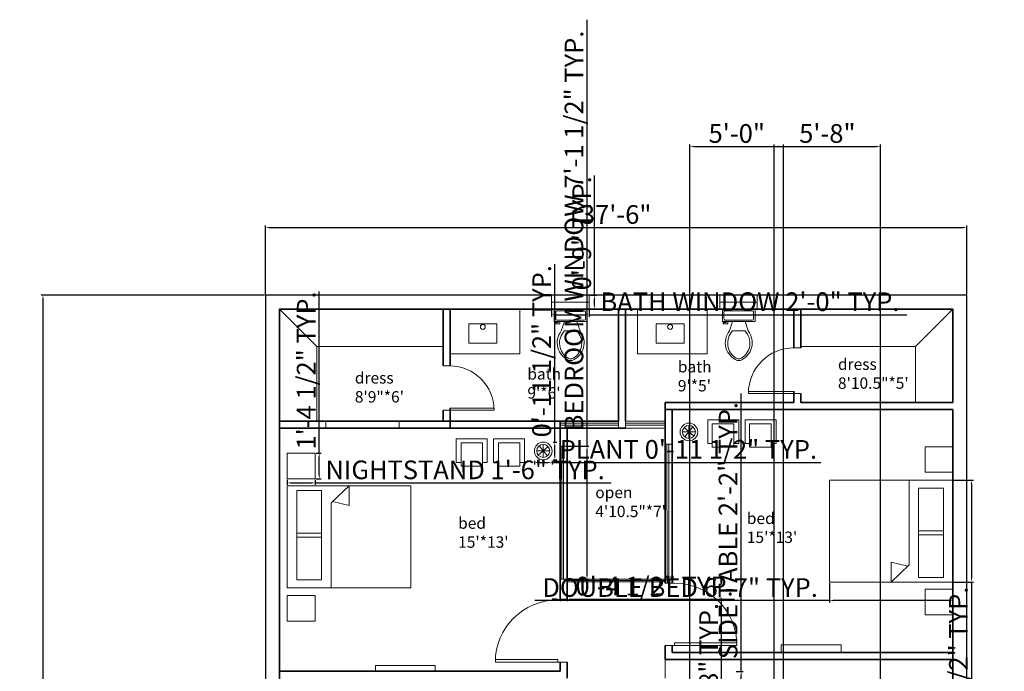
# Model space of a CAD drawing. Units: inches. Extents: x 3067 to 3879, y 3815 to 4813.
# Tile 3 of 3: x 3088 to 3719, y 4395 to 4813. Entities that reach past the tile are written whole.
import ezdxf

# ---------------------------------------------------------------- set-up
doc = ezdxf.new("R2010")
doc.units = ezdxf.units.IN
doc.linetypes.add('ACAD_ISO02W100', pattern=[15, 12, -3])
for name, color, linetype, lineweight in [('A-ANNO-DIMS', 2, 'Continuous', 18), ('A-AREA-IDEN', 7, 'Continuous', 18), ('A-DOOR', 3, 'Continuous', 18), ('A-EQPM', 8, 'Continuous', 18), ('A-FLOR-CASE', 8, 'Continuous', 20), ('A-FLOR-FIXT', 9, 'Continuous', 18), ('A-FLOR-OVHD', 8, 'ACAD_ISO02W100', 18), ('A-FURN', 8, 'Continuous', 18), ('A-GLAZ', 4, 'Continuous', 18), ('A-WALL', 7, 'Continuous', 35), ('C-PROP', 7, 'Continuous', 30)]:
    doc.layers.add(name, color=color, linetype=linetype, lineweight=lineweight)
doc.styles.get("Standard").update_dxf_attribs({"font": 'arial.ttf'})
doc.dimstyles.new('ISO-25', dxfattribs={"dimtxt": 12, "dimasz": 2.5, "dimexe": 1.25, "dimexo": 0.625, "dimtad": 1, "dimdec": 0, "dimlunit": 4, "dimtxsty": 'Standard', "dimcen": 2.5, "dimadec": 0, "dimazin": 0, "dimtfac": 1, "dimtdec": 0, "dimtmove": 0, "dimatfit": 3, "dimfxl": 1, "dimarcsym": 0})

# ---------------------------------------------------------------- blocks, each defined once
blk = doc.blocks.new('*U4')
for p, q in [((9.5, -6), (9.5, -2)), ((-10, -8.5), (-8, -8.5)), ((-10, -9.5), (-10, -8.5)), ((-7, -9.5), (-10, -9.5)), ((-8, -8.5), (-8, -8)), ((-7, -8), (-7, -9.5)), ((-4, -8), (-6, -14)), ((4, -8), (6, -14)), ((4, -14), (-4, -14))]:
    blk.add_line(p, q)
blk.add_lwpolyline([(10.5, -8), (10.5, 0), (-10.5, 0), (-10.5, -8)], close=True)
for points in [[(-9.5, -2), (-9.5, -6)], [(8.5, -1), (-8.5, -1)], [(-8.5, -7), (8.5, -7)]]:
    blk.add_lwpolyline(points)
for centre, radius, start, end in [((-8.62, -1.88), 0.884, 81.8699, 188.1301), ((-8.62, -6.12), 0.884, 171.8699, 278.1301), ((8.62, -1.88), 0.884, 351.8699, 98.1301), ((8.62, -6.12), 0.884, 261.8699, 8.1301), ((3.52, -21.58), 12.17, 141.46911, 247.97143), ((4.2, -21.82), 11.33, 136.36773, 238.94682), ((-3.52, -21.58), 12.17, 292.02843, 38.53071), ((-4.2, -21.82), 11.33, 301.05301, 43.63209), ((0, -27.88), 4, 245.73182, 294.26817), ((0, -29), 4, 254.86053, 285.13947)]:
    blk.add_arc(centre, radius, start, end)
blk = doc.blocks.new('*U2')
for p, q in [((0, 0), (0, -6)), ((40, 0), (40, -6))]:
    blk.add_line(p, q)
blk.add_lwpolyline([(0, 0), (0, 40), (1.75, 40), (1.75, 0)], close=True)
blk.add_arc((0, 0), 40, 0, 90)
blk = doc.blocks.new('*D7')
at = {"layer": 'A-ANNO-DIMS', "color": 0, "lineweight": -2, "transparency": 16777216}
for p, q in [((3245.41, 4636.9), (3245.41, 4680.99)), ((3695.41, 4636.9), (3695.41, 4680.99)), ((3247.91, 4679.74), (3692.91, 4679.74))]:
    blk.add_line(p, q, dxfattribs=at)
at = {"layer": 'A-ANNO-DIMS', "color": 0, "lineweight": 100, "transparency": 16777216}
for points in [[(3247.91, 4680.16), (3247.91, 4679.32), (3245.41, 4679.74)], [(3692.91, 4680.16), (3692.91, 4679.32), (3695.41, 4679.74)]]:
    blk.add_solid(points, dxfattribs=at)
at = {"layer": 'Defpoints', "color": 0, "lineweight": 100, "transparency": 16777216}
for p in [(3695.41, 4679.74), (3245.41, 4636.27), (3695.41, 4636.27)]:
    blk.add_point(p, dxfattribs=at)
at = {"layer": 'A-ANNO-DIMS', "color": 0, "transparency": 16777216, "insert": (3470.41, 4686.5), "char_height": 12, "attachment_point": 5}
blk.add_mtext('37\'-6"', dxfattribs=at)
blk = doc.blocks.new('*D8')
at = {"layer": 'A-ANNO-DIMS', "color": 0, "lineweight": -2, "transparency": 16777216}
for p, q in [((3244.78, 4636.27), (3101.49, 4636.27)), ((3102.74, 4633.77), (3102.74, 3918.77)), ((3244.78, 3916.27), (3101.49, 3916.27))]:
    blk.add_line(p, q, dxfattribs=at)
at = {"layer": 'A-ANNO-DIMS', "color": 0, "lineweight": 100, "transparency": 16777216}
for points in [[(3102.32, 4633.77), (3103.16, 4633.77), (3102.74, 4636.27)], [(3102.32, 3918.77), (3103.16, 3918.77), (3102.74, 3916.27)]]:
    blk.add_solid(points, dxfattribs=at)
at = {"layer": 'Defpoints', "color": 0, "lineweight": 100, "transparency": 16777216}
for p in [(3245.41, 4636.27), (3102.74, 3916.27), (3245.41, 3916.27)]:
    blk.add_point(p, dxfattribs=at)
at = {"layer": 'A-ANNO-DIMS', "color": 0, "transparency": 16777216, "insert": (3095.99, 4276.27), "char_height": 12, "attachment_point": 5, "rotation": 90}
blk.add_mtext("60'", dxfattribs=at)
blk = doc.blocks.new('CHAIR')
for p, q in [((0, 2.39), (0, 17.59)), ((0, 17.59), (19.86, 17.59)), ((19.86, 17.59), (19.86, 2.43)), ((3.13, 2.39), (0, 2.39)), ((19.86, 2.43), (16.92, 2.43))]:
    blk.add_line(p, q)
blk.add_lwpolyline([(3.13, 15.05), (16.92, 15.05), (16.92, 0), (3.13, 0)], close=True)
blk = doc.blocks.new('BED-DOUBLE')
for p, q in [((28.12, 54.48), (39.62, 65.45)), ((39.62, 65.45), (39.62, 52.71)), ((28.12, 0), (28.12, 54.48)), ((39.62, 52.71), (29.02, 55.33))]:
    blk.add_line(p, q)
for points in [[(0, 0), (79.24, 0), (79.24, 65.45), (0, 65.45)], [(6.11, 32.53), (21.99, 32.53), (21.99, 62.5), (6.11, 62.5)], [(6.11, 5.18), (21.99, 5.18), (21.99, 35.15), (6.11, 35.15)]]:
    blk.add_lwpolyline(points, close=True)
blk = doc.blocks.new('NIGHTSTAND')
blk.add_lwpolyline([(0, 0), (17.91, 0), (17.91, 16.38), (0, 16.38)], close=True)
blk = doc.blocks.new('PLANT-ROUND')
for p, q in [((1.02, 1.45), (7.33, 6.97)), ((6.87, 0.97), (1.63, 7.51)), ((4.2, 8.39), (4.2, 0)), ((0, 4.21), (8.39, 4.21))]:
    blk.add_line(p, q)
for radius in [5.68, 4.19]:
    blk.add_circle((4.19, 4.19), radius)
blk = doc.blocks.new('VANITY-BASIN')
for points in [[(0, 28.58), (44.74, 28.58), (44.74, 0), (0, 0)], [(11.93, 6.65), (29.93, 6.65), (29.93, 19.14), (11.93, 19.14)]]:
    blk.add_lwpolyline(points, close=True)
blk.add_circle((20.98, 17.18), 1.58)
blk = doc.blocks.new('WIN-BATH-24')
for p, q in [((0, 0), (0, 9)), ((24, 0), (24, 9)), ((0, 4.5), (24, 4.5))]:
    blk.add_line(p, q)
blk = doc.blocks.new('WIN-BEDROOM')
for p, q in [((1.09, 85.44), (1.21, 0)), ((2.25, 85.44), (2.25, 0))]:
    blk.add_line(p, q)
blk.add_lwpolyline([(0, 85.44), (4.5, 85.44), (4.5, 0), (0, 0)], close=True)
blk = doc.blocks.new('*D21')
at = {"layer": 'A-ANNO-DIMS', "color": 0, "lineweight": -2, "transparency": 16777216}
for p, q in [((3538.08, 4308.43), (3538.08, 4442)), ((3535.73, 4308.43), (3539.33, 4308.43)), ((3538.08, 4291.07), (3538.08, 4305.93)), ((3535.73, 4288.57), (3539.33, 4288.57))]:
    blk.add_line(p, q, dxfattribs=at)
at = {"layer": 'A-ANNO-DIMS', "color": 0, "lineweight": 100, "transparency": 16777216}
for points in [[(3537.67, 4305.93), (3538.5, 4305.93), (3538.08, 4308.43)], [(3537.67, 4291.07), (3538.5, 4291.07), (3538.08, 4288.57)]]:
    blk.add_solid(points, dxfattribs=at)
at = {"layer": 'Defpoints', "color": 0, "lineweight": 100, "transparency": 16777216}
for p in [(3535.11, 4308.43), (3538.08, 4308.43), (3535.11, 4288.57)]:
    blk.add_point(p, dxfattribs=at)
at = {"layer": 'A-ANNO-DIMS', "color": 0, "transparency": 16777216, "insert": (3531.25, 4376.46), "char_height": 12, "attachment_point": 5, "rotation": 90}
blk.add_mtext('CHAIR 1\'-8" TYP.', dxfattribs=at)
blk = doc.blocks.new('*D23')
at = {"layer": 'A-ANNO-DIMS', "color": 0, "lineweight": -2, "transparency": 16777216}
for p, q in [((3259.36, 4517.78), (3259.36, 4514.47)), ((3261.86, 4515.72), (3274.78, 4515.72)), ((3277.28, 4517.78), (3277.28, 4514.47)), ((3277.28, 4515.72), (3467.22, 4515.72))]:
    blk.add_line(p, q, dxfattribs=at)
at = {"layer": 'A-ANNO-DIMS', "color": 0, "lineweight": 100, "transparency": 16777216}
for points in [[(3261.86, 4516.13), (3261.86, 4515.3), (3259.36, 4515.72)], [(3274.78, 4516.13), (3274.78, 4515.3), (3277.28, 4515.72)]]:
    blk.add_solid(points, dxfattribs=at)
at = {"layer": 'Defpoints', "color": 0, "lineweight": 100, "transparency": 16777216}
for p in [(3259.36, 4518.4), (3277.28, 4518.4), (3277.28, 4515.72)]:
    blk.add_point(p, dxfattribs=at)
at = {"layer": 'A-ANNO-DIMS', "color": 0, "transparency": 16777216, "insert": (3373.5, 4522.55), "char_height": 12, "attachment_point": 5}
blk.add_mtext('NIGHTSTAND 1\'-6" TYP.', dxfattribs=at)
blk = doc.blocks.new('*D24')
at = {"layer": 'A-ANNO-DIMS', "color": 0, "lineweight": -2, "transparency": 16777216}
for p, q in [((3279.96, 4534.79), (3279.96, 4638.51)), ((3277.9, 4534.79), (3281.21, 4534.79)), ((3279.96, 4520.9), (3279.96, 4532.29)), ((3277.9, 4518.4), (3281.21, 4518.4))]:
    blk.add_line(p, q, dxfattribs=at)
at = {"layer": 'A-ANNO-DIMS', "color": 0, "lineweight": 100, "transparency": 16777216}
for points in [[(3279.55, 4532.29), (3280.38, 4532.29), (3279.96, 4534.79)], [(3279.55, 4520.9), (3280.38, 4520.9), (3279.96, 4518.4)]]:
    blk.add_solid(points, dxfattribs=at)
at = {"layer": 'Defpoints', "color": 0, "lineweight": 100, "transparency": 16777216}
for p in [(3277.28, 4534.79), (3279.96, 4534.79), (3277.28, 4518.4)]:
    blk.add_point(p, dxfattribs=at)
at = {"layer": 'A-ANNO-DIMS', "color": 0, "transparency": 16777216, "insert": (3273.13, 4587.9), "char_height": 12, "attachment_point": 5, "rotation": 90}
blk.add_mtext('1\'-4 1/2" TYP.', dxfattribs=at)
blk = doc.blocks.new('*D29')
at = {"layer": 'A-ANNO-DIMS', "color": 0, "lineweight": -2, "transparency": 16777216}
for p, q in [((3550.59, 4394.65), (3550.59, 4573.04)), ((3547.3, 4394.65), (3551.84, 4394.65)), ((3550.59, 4371.05), (3550.59, 4392.15)), ((3547.3, 4368.55), (3551.84, 4368.55))]:
    blk.add_line(p, q, dxfattribs=at)
at = {"layer": 'A-ANNO-DIMS', "color": 0, "lineweight": 100, "transparency": 16777216}
for points in [[(3550.17, 4392.15), (3551.01, 4392.15), (3550.59, 4394.65)], [(3550.17, 4371.05), (3551.01, 4371.05), (3550.59, 4368.55)]]:
    blk.add_solid(points, dxfattribs=at)
at = {"layer": 'Defpoints', "color": 0, "lineweight": 100, "transparency": 16777216}
for p in [(3546.67, 4394.65), (3550.59, 4394.65), (3546.67, 4368.55)]:
    blk.add_point(p, dxfattribs=at)
at = {"layer": 'A-ANNO-DIMS', "color": 0, "transparency": 16777216, "insert": (3543.76, 4485.1), "char_height": 12, "attachment_point": 5, "rotation": 90}
blk.add_mtext('SIDE TABLE 2\'-2" TYP.', dxfattribs=at)
blk = doc.blocks.new('*D35')
at = {"layer": 'A-ANNO-DIMS', "color": 0, "lineweight": -2, "transparency": 16777216}
for p, q in [((3607.17, 4451.42), (3607.17, 4438.91)), ((3686.41, 4451.42), (3686.41, 4438.91)), ((3607.17, 4440.16), (3418.14, 4440.16)), ((3683.91, 4440.16), (3609.67, 4440.16))]:
    blk.add_line(p, q, dxfattribs=at)
at = {"layer": 'A-ANNO-DIMS', "color": 0, "lineweight": 100, "transparency": 16777216}
for points in [[(3609.67, 4440.58), (3609.67, 4439.74), (3607.17, 4440.16)], [(3683.91, 4440.58), (3683.91, 4439.74), (3686.41, 4440.16)]]:
    blk.add_solid(points, dxfattribs=at)
at = {"layer": 'Defpoints', "color": 0, "lineweight": 100, "transparency": 16777216}
for p in [(3607.17, 4452.05), (3686.41, 4452.05), (3607.17, 4440.16)]:
    blk.add_point(p, dxfattribs=at)
at = {"layer": 'A-ANNO-DIMS', "color": 0, "transparency": 16777216, "insert": (3511.41, 4446.99), "char_height": 12, "attachment_point": 5}
blk.add_mtext('DOUBLE BED 6\'-7" TYP.', dxfattribs=at)
blk = doc.blocks.new('*D36')
at = {"layer": 'A-ANNO-DIMS', "color": 0, "lineweight": -2, "transparency": 16777216}
for p, q in [((3687.03, 4517.5), (3699.54, 4517.5)), ((3698.29, 4515), (3698.29, 4454.55)), ((3687.03, 4452.05), (3699.54, 4452.05)), ((3698.29, 4452.05), (3698.29, 4347.19))]:
    blk.add_line(p, q, dxfattribs=at)
at = {"layer": 'A-ANNO-DIMS', "color": 0, "lineweight": 100, "transparency": 16777216}
for points in [[(3697.88, 4515), (3698.71, 4515), (3698.29, 4517.5)], [(3697.88, 4454.55), (3698.71, 4454.55), (3698.29, 4452.05)]]:
    blk.add_solid(points, dxfattribs=at)
at = {"layer": 'Defpoints', "color": 0, "lineweight": 100, "transparency": 16777216}
for p in [(3686.41, 4517.5), (3686.41, 4452.05), (3698.29, 4452.05)]:
    blk.add_point(p, dxfattribs=at)
at = {"layer": 'A-ANNO-DIMS', "color": 0, "transparency": 16777216, "insert": (3691.46, 4398.37), "char_height": 12, "attachment_point": 5, "rotation": 90}
blk.add_mtext('5\'-5 1/2" TYP.', dxfattribs=at)
blk = doc.blocks.new('*D37')
at = {"layer": 'A-ANNO-DIMS', "color": 0, "lineweight": -2, "transparency": 16777216}
for p, q in [((3417.98, 4529.94), (3417.98, 4527.61)), ((3420.48, 4528.86), (3426.84, 4528.86)), ((3429.34, 4529.94), (3429.34, 4527.61)), ((3429.34, 4528.86), (3601.61, 4528.86))]:
    blk.add_line(p, q, dxfattribs=at)
at = {"layer": 'A-ANNO-DIMS', "color": 0, "lineweight": 100, "transparency": 16777216}
for points in [[(3420.48, 4529.28), (3420.48, 4528.44), (3417.98, 4528.86)], [(3426.84, 4529.28), (3426.84, 4528.44), (3429.34, 4528.86)]]:
    blk.add_solid(points, dxfattribs=at)
at = {"layer": 'Defpoints', "color": 0, "lineweight": 100, "transparency": 16777216}
for p in [(3417.98, 4530.56), (3429.34, 4530.56), (3429.34, 4528.86)]:
    blk.add_point(p, dxfattribs=at)
at = {"layer": 'A-ANNO-DIMS', "color": 0, "transparency": 16777216, "insert": (3516.72, 4535.69), "char_height": 12, "attachment_point": 5}
blk.add_mtext('PLANT 0\'-11 1/2" TYP.', dxfattribs=at)
blk = doc.blocks.new('*D38')
at = {"layer": 'A-ANNO-DIMS', "color": 0, "lineweight": -2, "transparency": 16777216}
for p, q in [((3431.04, 4541.92), (3431.04, 4656.1)), ((3429.96, 4541.92), (3432.29, 4541.92)), ((3431.04, 4533.06), (3431.04, 4539.42)), ((3429.96, 4530.56), (3432.29, 4530.56))]:
    blk.add_line(p, q, dxfattribs=at)
at = {"layer": 'A-ANNO-DIMS', "color": 0, "lineweight": 100, "transparency": 16777216}
for points in [[(3430.62, 4539.42), (3431.46, 4539.42), (3431.04, 4541.92)], [(3430.62, 4533.06), (3431.46, 4533.06), (3431.04, 4530.56)]]:
    blk.add_solid(points, dxfattribs=at)
at = {"layer": 'Defpoints', "color": 0, "lineweight": 100, "transparency": 16777216}
for p in [(3429.34, 4541.92), (3431.04, 4541.92), (3429.34, 4530.56)]:
    blk.add_point(p, dxfattribs=at)
at = {"layer": 'A-ANNO-DIMS', "color": 0, "transparency": 16777216, "insert": (3424.21, 4600.26), "char_height": 12, "attachment_point": 5, "rotation": 90}
blk.add_mtext('0\'-11 1/2" TYP.', dxfattribs=at)
blk = doc.blocks.new('*D39')
at = {"layer": 'A-ANNO-DIMS', "color": 0, "lineweight": -2, "transparency": 16777216}
for p, q in [((3429.01, 4626.65), (3429.01, 4622.42)), ((3431.51, 4623.67), (3450.51, 4623.67)), ((3453.01, 4626.65), (3453.01, 4622.42)), ((3453.01, 4623.67), (3656.95, 4623.67))]:
    blk.add_line(p, q, dxfattribs=at)
at = {"layer": 'A-ANNO-DIMS', "color": 0, "lineweight": 100, "transparency": 16777216}
for points in [[(3431.51, 4624.09), (3431.51, 4623.26), (3429.01, 4623.67)], [(3450.51, 4624.09), (3450.51, 4623.26), (3453.01, 4623.67)]]:
    blk.add_solid(points, dxfattribs=at)
at = {"layer": 'Defpoints', "color": 0, "lineweight": 100, "transparency": 16777216}
for p in [(3429.01, 4627.27), (3453.01, 4627.27), (3453.01, 4623.67)]:
    blk.add_point(p, dxfattribs=at)
at = {"layer": 'A-ANNO-DIMS', "color": 0, "transparency": 16777216, "insert": (3556.23, 4630.51), "char_height": 12, "attachment_point": 5}
blk.add_mtext('BATH WINDOW 2\'-0" TYP.', dxfattribs=at)
blk = doc.blocks.new('*D40')
at = {"layer": 'A-ANNO-DIMS', "color": 0, "lineweight": -2, "transparency": 16777216}
for p, q in [((3456.61, 4636.27), (3456.61, 4713.17)), ((3453.63, 4636.27), (3457.86, 4636.27)), ((3456.61, 4629.77), (3456.61, 4633.77)), ((3453.63, 4627.27), (3457.86, 4627.27))]:
    blk.add_line(p, q, dxfattribs=at)
at = {"layer": 'A-ANNO-DIMS', "color": 0, "lineweight": 100, "transparency": 16777216}
for points in [[(3456.19, 4633.77), (3457.03, 4633.77), (3456.61, 4636.27)], [(3456.19, 4629.77), (3457.03, 4629.77), (3456.61, 4627.27)]]:
    blk.add_solid(points, dxfattribs=at)
at = {"layer": 'Defpoints', "color": 0, "lineweight": 100, "transparency": 16777216}
for p in [(3453.01, 4636.27), (3456.61, 4636.27), (3453.01, 4627.27)]:
    blk.add_point(p, dxfattribs=at)
at = {"layer": 'A-ANNO-DIMS', "color": 0, "transparency": 16777216, "insert": (3449.86, 4675.97), "char_height": 12, "attachment_point": 5, "rotation": 90}
blk.add_mtext('0\'-9" TYP.', dxfattribs=at)
blk = doc.blocks.new('*D41')
at = {"layer": 'A-ANNO-DIMS', "color": 0, "lineweight": -2, "transparency": 16777216}
for p, q in [((3451.72, 4539.32), (3451.72, 4813.14)), ((3439.53, 4539.32), (3452.97, 4539.32)), ((3451.72, 4456.39), (3451.72, 4536.82)), ((3439.53, 4453.89), (3452.97, 4453.89))]:
    blk.add_line(p, q, dxfattribs=at)
at = {"layer": 'A-ANNO-DIMS', "color": 0, "lineweight": 100, "transparency": 16777216}
for points in [[(3451.31, 4536.82), (3452.14, 4536.82), (3451.72, 4539.32)], [(3451.31, 4456.39), (3452.14, 4456.39), (3451.72, 4453.89)]]:
    blk.add_solid(points, dxfattribs=at)
at = {"layer": 'Defpoints', "color": 0, "lineweight": 100, "transparency": 16777216}
for p in [(3438.91, 4539.32), (3451.72, 4539.32), (3438.91, 4453.89)]:
    blk.add_point(p, dxfattribs=at)
at = {"layer": 'A-ANNO-DIMS', "color": 0, "transparency": 16777216, "insert": (3444.89, 4677.48), "char_height": 12, "attachment_point": 5, "rotation": 90}
blk.add_mtext('BEDROOM WINDOW 7\'-1 1/2" TYP.', dxfattribs=at)
blk = doc.blocks.new('*D42')
at = {"layer": 'A-ANNO-DIMS', "color": 0, "lineweight": -2, "transparency": 16777216}
for p, q in [((3434.41, 4453.26), (3434.41, 4439.82)), ((3438.91, 4453.26), (3438.91, 4439.82)), ((3431.91, 4441.07), (3429.41, 4441.07)), ((3434.41, 4441.07), (3438.91, 4441.07)), ((3441.41, 4441.07), (3546.27, 4441.07))]:
    blk.add_line(p, q, dxfattribs=at)
at = {"layer": 'A-ANNO-DIMS', "color": 0, "lineweight": 100, "transparency": 16777216}
for points in [[(3431.91, 4441.49), (3431.91, 4440.65), (3434.41, 4441.07)], [(3441.41, 4441.49), (3441.41, 4440.65), (3438.91, 4441.07)]]:
    blk.add_solid(points, dxfattribs=at)
at = {"layer": 'Defpoints', "color": 0, "lineweight": 100, "transparency": 16777216}
for p in [(3434.41, 4453.89), (3438.91, 4453.89), (3438.91, 4441.07)]:
    blk.add_point(p, dxfattribs=at)
at = {"layer": 'A-ANNO-DIMS', "color": 0, "transparency": 16777216, "insert": (3495.09, 4447.9), "char_height": 12, "attachment_point": 5}
blk.add_mtext('0\'-4 1/2" TYP.', dxfattribs=at)
blk = doc.blocks.new('*D47')
at = {"layer": 'A-ANNO-DIMS', "color": 0, "lineweight": -2, "transparency": 16777216}
for p, q in [((3571.86, 4180.9), (3571.86, 4733.02)), ((3574.36, 4731.77), (3637.41, 4731.77)), ((3639.91, 4180.9), (3639.91, 4733.02))]:
    blk.add_line(p, q, dxfattribs=at)
at = {"layer": 'A-ANNO-DIMS', "color": 0, "lineweight": 100, "transparency": 16777216}
for points in [[(3574.36, 4732.19), (3574.36, 4731.36), (3571.86, 4731.77)], [(3637.41, 4732.19), (3637.41, 4731.36), (3639.91, 4731.77)]]:
    blk.add_solid(points, dxfattribs=at)
at = {"layer": 'Defpoints', "color": 0, "lineweight": 100, "transparency": 16777216}
for p in [(3639.91, 4731.77), (3571.86, 4180.27), (3639.91, 4180.27)]:
    blk.add_point(p, dxfattribs=at)
at = {"layer": 'A-ANNO-DIMS', "color": 0, "transparency": 16777216, "insert": (3605.89, 4738.52), "char_height": 12, "attachment_point": 5}
blk.add_mtext('5\'-8"', dxfattribs=at)
blk = doc.blocks.new('*D50')
at = {"layer": 'A-ANNO-DIMS', "color": 0, "lineweight": -2, "transparency": 16777216}
for p, q in [((3517.72, 4129.9), (3517.72, 4733.02)), ((3520.22, 4731.77), (3575.32, 4731.77)), ((3577.82, 4129.9), (3577.82, 4733.02))]:
    blk.add_line(p, q, dxfattribs=at)
at = {"layer": 'A-ANNO-DIMS', "color": 0, "lineweight": 100, "transparency": 16777216}
for points in [[(3520.22, 4732.19), (3520.22, 4731.36), (3517.72, 4731.77)], [(3575.32, 4732.19), (3575.32, 4731.36), (3577.82, 4731.77)]]:
    blk.add_solid(points, dxfattribs=at)
at = {"layer": 'Defpoints', "color": 0, "lineweight": 100, "transparency": 16777216}
for p in [(3577.82, 4731.77), (3517.72, 4129.27), (3577.82, 4129.27)]:
    blk.add_point(p, dxfattribs=at)
at = {"layer": 'A-ANNO-DIMS', "color": 0, "transparency": 16777216, "insert": (3547.77, 4738.52), "char_height": 12, "attachment_point": 5}
blk.add_mtext('5\'-0"', dxfattribs=at)

msp = doc.modelspace()

# ---------------------------------------------------------------- linework, layer by layer
at = {"layer": 'A-EQPM'}
for points in [[(3576.16, 4406.77), (3614.64, 4406.77), (3614.64, 4411.85), (3576.16, 4411.85)], [(3316.12, 4394.77), (3354.25, 4394.77), (3354.25, 4398.57), (3316.12, 4398.57)]]:
    msp.add_lwpolyline(points, close=True, dxfattribs=at)
at = {"layer": 'A-FLOR-CASE'}
for p, q in [((3278.41, 4603.27), (3254.41, 4627.27)), ((3359.41, 4627.27), (3359.41, 4603.27)), ((3588.91, 4627.27), (3588.91, 4603.27)), ((3662.41, 4603.27), (3686.41, 4627.27)), ((3278.41, 4555.6), (3278.41, 4603.27)), ((3359.41, 4603.27), (3278.41, 4603.27)), ((3588.91, 4603.27), (3662.41, 4603.27)), ((3662.41, 4567.27), (3662.41, 4603.27)), ((3686.41, 4567.27), (3662.41, 4567.27)), ((3278.41, 4556.68), (3278.41, 4555.27))]:
    msp.add_line(p, q, dxfattribs=at)
at = {"layer": 'A-FLOR-OVHD'}
msp.add_line((3501.91, 4402.27), (3501.91, 4222.27), dxfattribs=at)
at = {"layer": 'A-GLAZ'}
for p, q in [((3434.41, 4554.04), (3471.91, 4554.04)), ((3471.91, 4555.27), (3471.91, 4550.77)), ((3476.41, 4555.27), (3501.91, 4555.27)), ((3476.41, 4555.27), (3476.41, 4550.77)), ((3476.41, 4554.04), (3501.91, 4554.04)), ((3434.41, 4552.83), (3471.91, 4552.83)), ((3476.41, 4552.83), (3501.91, 4552.83)), ((3476.41, 4550.77), (3501.91, 4550.77)), ((3438.91, 4453.05), (3501.91, 4453.05))]:
    msp.add_line(p, q, dxfattribs=at)
for points in [[(3284.1, 4555.27), (3331.23, 4555.27), (3331.23, 4550.77), (3284.1, 4550.77)], [(3501.91, 4452.21), (3438.91, 4452.21), (3438.91, 4453.89), (3501.91, 4453.89)]]:
    msp.add_lwpolyline(points, close=True, dxfattribs=at)
at = {"layer": 'A-WALL'}
for p, q in [((3254.41, 4627.27), (3359.41, 4627.27)), ((3359.41, 4627.27), (3359.41, 4590.85)), ((3363.91, 4627.27), (3363.91, 4590.85)), ((3363.91, 4627.27), (3471.91, 4627.27)), ((3471.91, 4627.27), (3471.91, 4555.27)), ((3476.41, 4627.27), (3476.41, 4555.27)), ((3476.41, 4627.27), (3584.41, 4627.27)), ((3584.41, 4627.27), (3584.41, 4602.48)), ((3588.91, 4627.27), (3588.91, 4602.48)), ((3588.91, 4627.27), (3686.41, 4627.27)), ((3584.41, 4574.48), (3584.41, 4567.27)), ((3588.91, 4573.2), (3588.91, 4567.27)), ((3584.41, 4567.27), (3501.91, 4567.27)), ((3501.91, 4562.77), (3501.91, 4567.27)), ((3588.91, 4567.27), (3686.41, 4567.27)), ((3359.41, 4562.42), (3359.41, 4555.27)), ((3363.91, 4563.66), (3363.91, 4550.77)), ((3588.91, 4562.77), (3501.91, 4562.77)), ((3501.91, 4451.29), (3501.91, 4562.77)), ((3506.41, 4451.29), (3506.41, 4562.77)), ((3588.91, 4562.77), (3686.41, 4562.77)), ((3686.41, 4562.77), (3686.41, 4406.77)), ((3359.41, 4555.27), (3254.41, 4555.27)), ((3471.91, 4555.27), (3359.41, 4555.27)), ((3434.41, 4545.06), (3434.41, 4555.27)), ((3363.91, 4550.77), (3254.41, 4550.77)), ((3254.41, 4550.77), (3254.41, 4394.77)), ((3476.41, 4550.77), (3359.41, 4550.77)), ((3434.41, 4440.62), (3434.41, 4550.77)), ((3438.91, 4440.62), (3438.91, 4550.77)), ((3501.91, 4402.27), (3501.91, 4411.29)), ((3506.41, 4406.77), (3506.41, 4411.29)), ((3686.41, 4402.27), (3501.91, 4402.27)), ((3686.41, 4406.77), (3506.41, 4406.77)), ((3686.41, 4402.27), (3686.41, 4222.27)), ((3434.41, 4394.77), (3434.41, 4400.62)), ((3438.91, 4390.27), (3438.91, 4400.62)), ((3254.41, 4394.77), (3422.41, 4394.77)), ((3254.41, 4394.77), (3434.41, 4394.77))]:
    msp.add_line(p, q, dxfattribs=at)
for points in [[(3686.41, 4567.27), (3686.41, 4627.27), (3254.41, 4627.27), (3254.41, 3925.27), (3494.41, 3925.27)], [(3686.41, 3925.27), (3686.41, 4562.77)]]:
    msp.add_lwpolyline(points, dxfattribs=at)
at = {"layer": 'C-PROP'}
msp.add_lwpolyline([(3245.41, 3916.27), (3695.41, 3916.27), (3695.41, 4636.27), (3245.41, 4636.27)], close=True, dxfattribs=at)

# ---------------------------------------------------------------- block references
at = {"layer": 'A-DOOR'}
for p, xscale, yscale, zscale, rotation in [((3584.52, 4573.2), 0.7320240099699031, 0.7320240099699031, 0.7320240099699031, 90), ((3363.67, 4562.42), -0.7108348998799947, 0.7108348998799947, 0.7108348998799947, 270)]:
    msp.add_blockref('*U2', p, dxfattribs=dict(at, xscale=xscale, yscale=yscale, zscale=zscale, rotation=rotation))
at = {"layer": 'A-DOOR', "xscale": -1, "rotation": 270}
msp.add_blockref('*U2', (3507.91, 4411.29), dxfattribs=at)
at = {"layer": 'A-DOOR', "rotation": 90}
msp.add_blockref('*U2', (3432.91, 4400.62), dxfattribs=at)
at = {"layer": 'A-FLOR-FIXT'}
for name, p in [('VANITY-BASIN', (3363.91, 4598.69)), ('*U4', (3441.22, 4627.27)), ('VANITY-BASIN', (3484.04, 4598.69)), ('*U4', (3549.06, 4627.27))]:
    msp.add_blockref(name, p, dxfattribs=at)
at = {"layer": 'A-FURN', "extrusion": (0, 0, -1), "zscale": -1}
for name, p in [('PLANT-ROUND', (-3521.3, 4544.24)), ('CHAIR', (-3549, 4538.6)), ('CHAIR', (-3572.95, 4538.6))]:
    msp.add_blockref(name, p, dxfattribs=at)
at = {"layer": 'A-FURN'}
for name, p in [('CHAIR', (3367.81, 4526.4)), ('CHAIR', (3391.76, 4526.4)), ('PLANT-ROUND', (3419.46, 4532.05)), ('NIGHTSTAND', (3259.36, 4518.4)), ('BED-DOUBLE', (3259.43, 4448.4)), ('NIGHTSTAND', (3259.36, 4426.98))]:
    msp.add_blockref(name, p, dxfattribs=at)
at = {"layer": 'A-FURN', "rotation": 180}
for name, p in [('NIGHTSTAND', (3686.47, 4538.92)), ('BED-DOUBLE', (3686.41, 4517.5)), ('NIGHTSTAND', (3686.47, 4447.5))]:
    msp.add_blockref(name, p, dxfattribs=at)
at = {"layer": 'A-GLAZ'}
for name, p in [('WIN-BATH-24', (3429.01, 4627.27)), ('WIN-BATH-24', (3536.92, 4627.27)), ('WIN-BEDROOM', (3434.41, 4453.89)), ('WIN-BEDROOM', (3501.91, 4455.14))]:
    msp.add_blockref(name, p, dxfattribs=at)

# ---------------------------------------------------------------- texts
at = {"layer": 'A-AREA-IDEN', "char_height": 7.308, "attachment_point": 1}
for s, insert in [("bath\\P9'*5'", (3509.98, 4593.95)), ('dress\\P8\'10.5"*5\'', (3612.67, 4595.61)), ('dress\\P8\'9"*6\'', (3302.78, 4586.82)), ("bath\\P9'*6'", (3413.46, 4589.34)), ('open\\P4\'10.5"*7\'', (3457.02, 4513.24)), ("bed\\P15'*13'", (3554.23, 4496.64)), ("bed\\P15'*13'", (3369.05, 4493.57))]:
    msp.add_mtext_dynamic_manual_height_columns(s, width=269.495, gutter_width=36.54, heights=[0], dxfattribs=dict(at, insert=insert))

# ---------------------------------------------------------------- dimensions: what is measured, and where the dimension line sits
at = {"layer": 'A-ANNO-DIMS'}
for base, p1, p2, angle, text, picture, middle in [((3451.72, 4539.32), (3438.91, 4453.89), (3438.91, 4539.32), 90, 'BEDROOM WINDOW <> TYP.', '*D41', (3444.89, 4677.48)), ((3456.61, 4636.27), (3453.01, 4627.27), (3453.01, 4636.27), 90, '<> TYP.', '*D40', (3449.86, 4675.97)), ((3431.04, 4541.92), (3429.34, 4530.56), (3429.34, 4541.92), 90, '<> TYP.', '*D38', (3424.21, 4600.26)), ((3279.96, 4534.79), (3277.28, 4518.4), (3277.28, 4534.79), 90, '<> TYP.', '*D24', (3273.13, 4587.9)), ((3550.59, 4394.65), (3546.67, 4368.55), (3546.67, 4394.65), 90, 'SIDE TABLE <> TYP.', '*D29', (3543.76, 4485.1)), ((3698.2935, 4452.0456), (3686.4073, 4517.4994), (3686.4073, 4452.0456), 270, '<> TYP.', '*D36', (3691.4639, 4398.3667)), ((3607.17, 4440.16), (3686.41, 4452.05), (3607.17, 4452.05), 180, 'DOUBLE BED <> TYP.', '*D35', (3511.41, 4446.99)), ((3538.08, 4308.43), (3535.11, 4288.57), (3535.11, 4308.43), 90, 'CHAIR <> TYP.', '*D21', (3531.25, 4376.46))]:
    dim = msp.add_linear_dim(base=base, p1=p1, p2=p2, angle=angle, text=text, dimstyle='ISO-25', override={"dimdec": 1, "dimlfac": 1, "dimrnd": 0, "dimzin": 1, "dimdsep": 46, "dimlunit": 4, "dimfrac": 2}, dxfattribs=at)
    dim.commit()
    dim.dimension.update_dxf_attribs({"geometry": picture, "text_midpoint": middle})
for base, p1, p2, override, picture, middle in [((3577.82, 4731.77), (3517.72, 4129.27), (3577.82, 4129.27), {"dimdec": 1, "dimlfac": 1, "dimrnd": 0, "dimzin": 1, "dimdsep": 46, "dimlunit": 4, "dimfrac": 2}, '*D50', (3547.77, 4738.52)), ((3639.9073, 4731.7725), (3571.865, 4180.2725), (3639.9073, 4180.2725), {"dimdec": 1, "dimlfac": 1, "dimrnd": 0, "dimzin": 1, "dimdsep": 46, "dimlunit": 4, "dimfrac": 2}, '*D47', (3605.8862, 4738.5244)), ((3695.41, 4679.74), (3245.41, 4636.27), (3695.41, 4636.27), {"dimclrd": 0, "dimclre": 0, "dimclrt": 0}, '*D7', (3470.41, 4686.5))]:
    dim = msp.add_linear_dim(base=base, p1=p1, p2=p2, dimstyle='ISO-25', override=override, dxfattribs=at)
    dim.commit()
    dim.dimension.update_dxf_attribs({"geometry": picture, "text_midpoint": middle})
for base, p1, p2, text, picture, middle in [((3453.01, 4623.67), (3429.01, 4627.27), (3453.01, 4627.27), 'BATH WINDOW <> TYP.', '*D39', (3556.23, 4630.51)), ((3429.34, 4528.86), (3417.98, 4530.56), (3429.34, 4530.56), 'PLANT <> TYP.', '*D37', (3516.72, 4535.69)), ((3277.28, 4515.72), (3259.36, 4518.4), (3277.28, 4518.4), 'NIGHTSTAND <> TYP.', '*D23', (3373.5, 4522.55)), ((3438.91, 4441.07), (3434.41, 4453.89), (3438.91, 4453.89), '<> TYP.', '*D42', (3495.09, 4447.9))]:
    dim = msp.add_linear_dim(base=base, p1=p1, p2=p2, text=text, dimstyle='ISO-25', override={"dimdec": 1, "dimlfac": 1, "dimrnd": 0, "dimzin": 1, "dimdsep": 46, "dimlunit": 4, "dimfrac": 2}, dxfattribs=at)
    dim.commit()
    dim.dimension.update_dxf_attribs({"geometry": picture, "text_midpoint": middle})
dim = msp.add_linear_dim(base=(3102.74, 3916.27), p1=(3245.41, 4636.27), p2=(3245.41, 3916.27), angle=90, dimstyle='ISO-25', override={"dimclrd": 0, "dimclre": 0, "dimclrt": 0}, dxfattribs=at)
dim.commit()
dim.dimension.update_dxf_attribs({"geometry": '*D8', "text_midpoint": (3095.99, 4276.27)})

doc.saveas('drawing.dxf')
